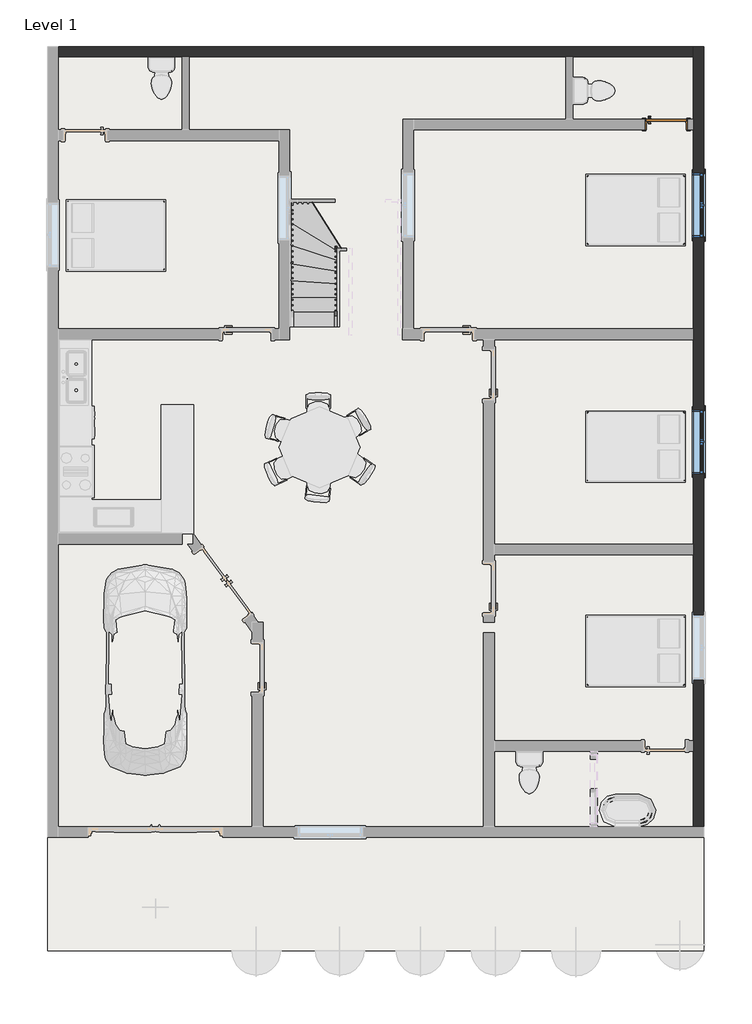
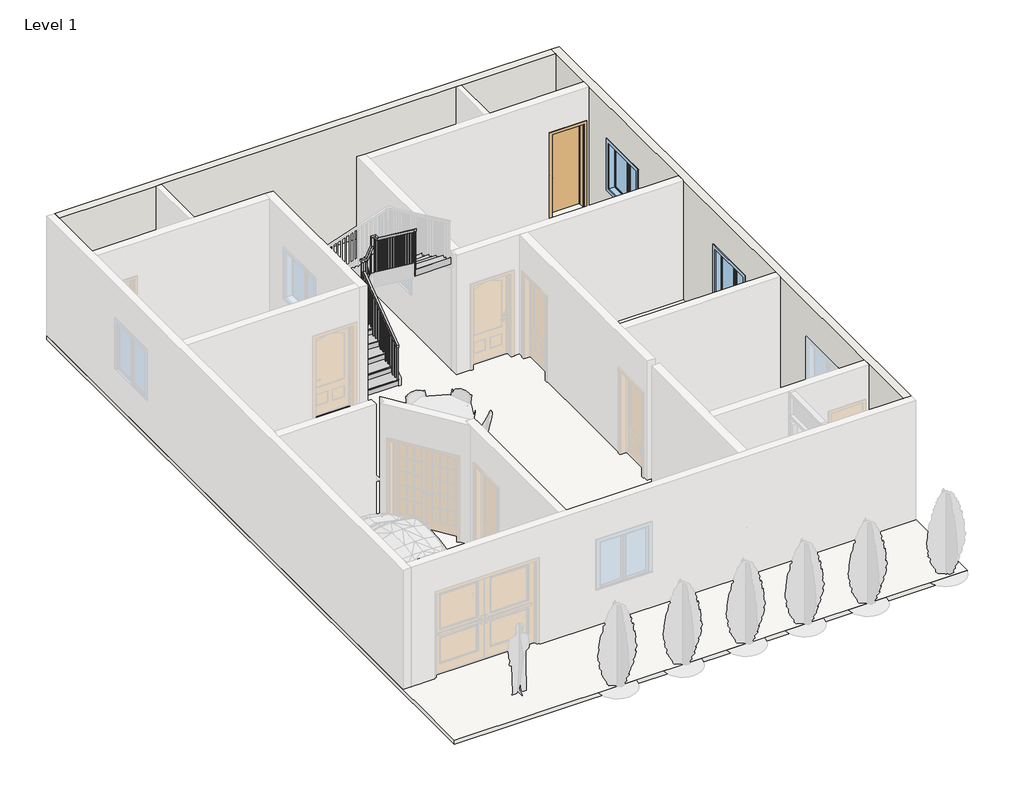
# One storey, part 2 of 3: 2 walls, 2 windows, 1 door, 1 railing, 1 slab, 1 stair flight.
"""IFC4 building model written with IfcOpenShell, lengths in millimetres."""

from ifc_helpers import new_model, si_unit, frame, origin, place, context, project, spatial, polyline, outline, extrude, faceted_brep, transform, mapped, element, save
from components import door_715cd483, stair_flight_58ce975e, window_d2c79e1c

model = new_model("IFC4")

# Units and contexts
model_context = context("Model", 3, world=origin())
ifc_project = project(units=[si_unit("LENGTHUNIT", "METRE", prefix="MILLI")], contexts=[model_context])

# Site, building, storey
site = spatial("IfcSite", under=ifc_project)
building = spatial("IfcBuilding", under=site)
storey = spatial("IfcBuildingStorey", under=building, Name="Level 1", Elevation=0.0)

# Door
placement = place(None, origin())
door_shape = door_715cd483(model_context)
element("IfcDoor", 1, ObjectType="Door-Interior-Single-Flush_Panel-Wood : 30\" x 84\"", at=placement, inside=storey, context=model_context, shape_type="MappedRepresentation", body=[
    mapped(door_shape, transform((9115.2875253, 6893.0277309, 0.0), x_axis=(1.0, 0.0, 0.0), y_axis=(0.0, 1.0, 0.0), z_axis=(0.0, 0.0, 1.0))),
])

# Railing
element("IfcRailing", 2, ObjectType="Handrail - Rectangular", at=placement, inside=storey, context=model_context, shape_type="SolidModel", body=[
    faceted_brep([(2841.0207007, 3072.6312797, 1047.851748), (2841.0207007, 3072.6312797, 984.8215118), (2891.8207007, 3072.6312797, 984.8215118), (2891.8207007, 3072.6312797, 1047.851748), (2841.0207007, 4480.7853358, 2082.1188207), (2841.0207007, 4531.5853358, 2056.4003879), (2891.8207007, 4531.5853358, 2056.4003879), (2891.8207007, 4480.7853358, 2082.1188207), (2841.0207007, 4480.7853358, 2326.0056881), (2841.0207007, 4531.5853358, 2275.2056881), (2891.8207007, 4531.5853358, 2275.2056881), (2891.8207007, 4480.7853358, 2326.0056881), (2841.0207007, 4607.7853358, 2326.0056881), (2841.0207007, 4607.7853358, 2275.2056881), (2891.8207007, 4556.9853358, 2275.2056881), (2891.8207007, 4556.9853358, 2326.0056881), (2968.0207007, 4607.7853358, 2326.0056881), (3000.34384, 4607.7853358, 2275.2056881), (3000.34384, 4556.9853358, 2275.2056881), (2968.0207007, 4556.9853358, 2326.0056881), (3095.0207007, 4607.7853358, 2597.5625884), (3145.8207007, 4607.7853358, 2586.2706121), (3145.8207007, 4556.9853358, 2586.2706121), (3095.0207007, 4556.9853358, 2597.5625884), (3095.0207007, 4607.7853358, 2827.5043941), (3145.8207007, 4607.7853358, 2776.7043941), (3145.8207007, 4556.9853358, 2776.7043941), (3095.0207007, 4556.9853358, 2827.5043941), (3222.0207007, 4607.7853358, 2827.5043941), (3222.0207007, 4607.7853358, 2776.7043941), (3171.2207007, 4556.9853358, 2776.7043941), (3171.2207007, 4556.9853358, 2827.5043941), (3222.0207007, 4480.7853358, 2827.5043941), (3222.0207007, 4463.8549082, 2776.7043941), (3171.2207007, 4463.8549082, 2776.7043941), (3171.2207007, 4480.7853358, 2827.5043941), (3222.0207007, 2913.6927876, 4002.5717223), (3171.2207007, 2913.6927876, 4002.5717223), (3171.2207007, 2913.6927876, 3939.076625), (3222.0207007, 2913.6927876, 3939.076625)], [[[0, 1, 2, 3]], [[1, 0, 4, 5]], [[2, 1, 5, 6]], [[3, 2, 6, 7]], [[0, 3, 7, 4]], [[5, 4, 8, 9]], [[6, 5, 9, 10]], [[7, 6, 10, 11]], [[4, 7, 11, 8]], [[9, 8, 12, 13]], [[10, 9, 13, 14]], [[11, 10, 14, 15]], [[8, 11, 15, 12]], [[13, 12, 16, 17]], [[14, 13, 17, 18]], [[15, 14, 18, 19]], [[12, 15, 19, 16]], [[17, 16, 20, 21]], [[18, 17, 21, 22]], [[19, 18, 22, 23]], [[16, 19, 23, 20]], [[21, 20, 24, 25]], [[22, 21, 25, 26]], [[23, 22, 26, 27]], [[20, 23, 27, 24]], [[25, 24, 28, 29]], [[26, 25, 29, 30]], [[27, 26, 30, 31]], [[24, 27, 31, 28]], [[29, 28, 32, 33]], [[30, 29, 33, 34]], [[31, 30, 34, 35]], [[28, 31, 35, 32]], [[36, 37, 38, 39]], [[33, 32, 36, 39]], [[34, 33, 39, 38]], [[35, 34, 38, 37]], [[32, 35, 37, 36]]]),
    extrude(outline(polyline([(2904.9263419, 3945.6500491), (2923.9763419, 3931.3656135), (2923.9763419, 2878.6666667), (2904.9263419, 2878.6666667), (2904.9263419, 3945.6500491)])), frame((3187.0957007, 0.0, 0.0), z_axis=(1.0, 0.0, 0.0), x_axis=(0.0, 1.0, 0.0)), (0.0, 0.0, 1.0), 19.05),
    extrude(outline(polyline([(3006.5263419, 3869.4663925), (3025.5763419, 3855.1819569), (3025.5763419, 2878.6666667), (3006.5263419, 2878.6666667), (3006.5263419, 3869.4663925)])), frame((3187.0957007, 0.0, 0.0), z_axis=(1.0, 0.0, 0.0), x_axis=(0.0, 1.0, 0.0)), (0.0, 0.0, 1.0), 19.05),
    extrude(outline(polyline([(3108.1263419, 3793.2827359), (3127.1763419, 3778.9983003), (3127.1763419, 2878.6666667), (3108.1263419, 2878.6666667), (3108.1263419, 3793.2827359)])), frame((3187.0957007, 0.0, 0.0), z_axis=(1.0, 0.0, 0.0), x_axis=(0.0, 1.0, 0.0)), (0.0, 0.0, 1.0), 19.05),
    extrude(outline(polyline([(3209.7263419, 3717.0990793), (3228.7763419, 3702.8146437), (3228.7763419, 2709.3333333), (3209.7263419, 2709.3333333), (3209.7263419, 3717.0990793)])), frame((3187.0957007, 0.0, 0.0), z_axis=(1.0, 0.0, 0.0), x_axis=(0.0, 1.0, 0.0)), (0.0, 0.0, 1.0), 19.05),
    extrude(outline(polyline([(3311.3263419, 3640.9154227), (3330.3763419, 3626.6309871), (3330.3763419, 2709.3333333), (3311.3263419, 2709.3333333), (3311.3263419, 3640.9154227)])), frame((3187.0957007, 0.0, 0.0), z_axis=(1.0, 0.0, 0.0), x_axis=(0.0, 1.0, 0.0)), (0.0, 0.0, 1.0), 19.05),
    extrude(outline(polyline([(3412.9263419, 3564.7317661), (3431.9763419, 3550.4473305), (3431.9763419, 2709.3333333), (3412.9263419, 2709.3333333), (3412.9263419, 3564.7317661)])), frame((3187.0957007, 0.0, 0.0), z_axis=(1.0, 0.0, 0.0), x_axis=(0.0, 1.0, 0.0)), (0.0, 0.0, 1.0), 19.05),
    extrude(outline(polyline([(3514.5263419, 3488.5481095), (3533.5763419, 3474.2636739), (3533.5763419, 2540.0), (3514.5263419, 2540.0), (3514.5263419, 3488.5481095)])), frame((3187.0957007, 0.0, 0.0), z_axis=(1.0, 0.0, 0.0), x_axis=(0.0, 1.0, 0.0)), (0.0, 0.0, 1.0), 19.05),
    extrude(outline(polyline([(3616.1263419, 3412.3644529), (3635.1763419, 3398.0800173), (3635.1763419, 2540.0), (3616.1263419, 2540.0), (3616.1263419, 3412.3644529)])), frame((3187.0957007, 0.0, 0.0), z_axis=(1.0, 0.0, 0.0), x_axis=(0.0, 1.0, 0.0)), (0.0, 0.0, 1.0), 19.05),
    extrude(outline(polyline([(3717.7263419, 3336.1807963), (3736.7763419, 3321.8963607), (3736.7763419, 2370.6666667), (3717.7263419, 2370.6666667), (3717.7263419, 3336.1807963)])), frame((3187.0957007, 0.0, 0.0), z_axis=(1.0, 0.0, 0.0), x_axis=(0.0, 1.0, 0.0)), (0.0, 0.0, 1.0), 19.05),
    extrude(outline(polyline([(3819.3263419, 3259.9971397), (3838.3763419, 3245.7127041), (3838.3763419, 2370.6666667), (3819.3263419, 2370.6666667), (3819.3263419, 3259.9971397)])), frame((3187.0957007, 0.0, 0.0), z_axis=(1.0, 0.0, 0.0), x_axis=(0.0, 1.0, 0.0)), (0.0, 0.0, 1.0), 19.05),
    extrude(outline(polyline([(3920.9263419, 3183.8134831), (3939.9763419, 3169.5290475), (3939.9763419, 2370.6666667), (3920.9263419, 2370.6666667), (3920.9263419, 3183.8134831)])), frame((3187.0957007, 0.0, 0.0), z_axis=(1.0, 0.0, 0.0), x_axis=(0.0, 1.0, 0.0)), (0.0, 0.0, 1.0), 19.05),
    extrude(outline(polyline([(4022.5263419, 3107.6298265), (4041.5763419, 3093.3453909), (4041.5763419, 2201.3333333), (4022.5263419, 2201.3333333), (4022.5263419, 3107.6298265)])), frame((3187.0957007, 0.0, 0.0), z_axis=(1.0, 0.0, 0.0), x_axis=(0.0, 1.0, 0.0)), (0.0, 0.0, 1.0), 19.05),
    extrude(outline(polyline([(4124.1263419, 3031.4461699), (4143.1763419, 3017.1617343), (4143.1763419, 2201.3333333), (4124.1263419, 2201.3333333), (4124.1263419, 3031.4461699)])), frame((3187.0957007, 0.0, 0.0), z_axis=(1.0, 0.0, 0.0), x_axis=(0.0, 1.0, 0.0)), (0.0, 0.0, 1.0), 19.05),
    extrude(outline(polyline([(4225.7263419, 2955.2625133), (4244.7763419, 2940.9780777), (4244.7763419, 2032.0), (4225.7263419, 2032.0), (4225.7263419, 2955.2625133)])), frame((3187.0957007, 0.0, 0.0), z_axis=(1.0, 0.0, 0.0), x_axis=(0.0, 1.0, 0.0)), (0.0, 0.0, 1.0), 19.05),
    extrude(outline(polyline([(4327.3263419, 2879.0788567), (4346.3763419, 2864.7944211), (4346.3763419, 2032.0), (4327.3263419, 2032.0), (4327.3263419, 2879.0788567)])), frame((3187.0957007, 0.0, 0.0), z_axis=(1.0, 0.0, 0.0), x_axis=(0.0, 1.0, 0.0)), (0.0, 0.0, 1.0), 19.05),
    extrude(outline(polyline([(4428.9263419, 2802.8952001), (4447.9763419, 2788.6107645), (4447.9763419, 1862.6666667), (4428.9263419, 1862.6666667), (4428.9263419, 2802.8952001)])), frame((3187.0957007, 0.0, 0.0), z_axis=(1.0, 0.0, 0.0), x_axis=(0.0, 1.0, 0.0)), (0.0, 0.0, 1.0), 19.05),
    extrude(outline(polyline([(2467.6943692, 3090.3657193), (2426.9608342, 3071.3157193), (1524.0, 3071.3157193), (1524.0, 3090.3657193), (2467.6943692, 3090.3657193)])), frame((0.0, 4572.8603358, 0.0), z_axis=(0.0, 1.0, 0.0), x_axis=(0.0, 0.0, 1.0)), (0.0, 0.0, 1.0), 19.05),
    extrude(outline(polyline([(2250.448849, 2988.7657193), (2209.7153139, 2969.7157193), (1354.6666667, 2969.7157193), (1354.6666667, 2988.7657193), (2250.448849, 2988.7657193)])), frame((0.0, 4572.8603358, 0.0), z_axis=(0.0, 1.0, 0.0), x_axis=(0.0, 0.0, 1.0)), (0.0, 0.0, 1.0), 19.05),
    extrude(outline(polyline([(4485.5062797, 2022.5560437), (4504.5562797, 2036.54797), (4504.5562797, 1016.0), (4485.5062797, 1016.0), (4485.5062797, 2022.5560437)])), frame((2856.8957007, 0.0, 0.0), z_axis=(1.0, 0.0, 0.0), x_axis=(0.0, 1.0, 0.0)), (0.0, 0.0, 1.0), 19.05),
    extrude(outline(polyline([(4383.9062797, 1947.9324369), (4402.9562797, 1961.9243632), (4402.9562797, 1016.0), (4383.9062797, 1016.0), (4383.9062797, 1947.9324369)])), frame((2856.8957007, 0.0, 0.0), z_axis=(1.0, 0.0, 0.0), x_axis=(0.0, 1.0, 0.0)), (0.0, 0.0, 1.0), 19.05),
    extrude(outline(polyline([(4282.3062797, 1873.3088301), (4301.3562797, 1887.3007564), (4301.3562797, 846.6666667), (4282.3062797, 846.6666667), (4282.3062797, 1873.3088301)])), frame((2856.8957007, 0.0, 0.0), z_axis=(1.0, 0.0, 0.0), x_axis=(0.0, 1.0, 0.0)), (0.0, 0.0, 1.0), 19.05),
    extrude(outline(polyline([(4180.7062797, 1798.6852234), (4199.7562797, 1812.6771496), (4199.7562797, 846.6666667), (4180.7062797, 846.6666667), (4180.7062797, 1798.6852234)])), frame((2856.8957007, 0.0, 0.0), z_axis=(1.0, 0.0, 0.0), x_axis=(0.0, 1.0, 0.0)), (0.0, 0.0, 1.0), 19.05),
    extrude(outline(polyline([(4079.1062797, 1724.0616166), (4098.1562797, 1738.0535428), (4098.1562797, 677.3333333), (4079.1062797, 677.3333333), (4079.1062797, 1724.0616166)])), frame((2856.8957007, 0.0, 0.0), z_axis=(1.0, 0.0, 0.0), x_axis=(0.0, 1.0, 0.0)), (0.0, 0.0, 1.0), 19.05),
    extrude(outline(polyline([(3977.5062797, 1649.4380098), (3996.5562797, 1663.429936), (3996.5562797, 677.3333333), (3977.5062797, 677.3333333), (3977.5062797, 1649.4380098)])), frame((2856.8957007, 0.0, 0.0), z_axis=(1.0, 0.0, 0.0), x_axis=(0.0, 1.0, 0.0)), (0.0, 0.0, 1.0), 19.05),
    extrude(outline(polyline([(3875.9062797, 1574.814403), (3894.9562797, 1588.8063293), (3894.9562797, 677.3333333), (3875.9062797, 677.3333333), (3875.9062797, 1574.814403)])), frame((2856.8957007, 0.0, 0.0), z_axis=(1.0, 0.0, 0.0), x_axis=(0.0, 1.0, 0.0)), (0.0, 0.0, 1.0), 19.05),
    extrude(outline(polyline([(3774.3062797, 1500.1907962), (3793.3562797, 1514.1827225), (3793.3562797, 508.0), (3774.3062797, 508.0), (3774.3062797, 1500.1907962)])), frame((2856.8957007, 0.0, 0.0), z_axis=(1.0, 0.0, 0.0), x_axis=(0.0, 1.0, 0.0)), (0.0, 0.0, 1.0), 19.05),
    extrude(outline(polyline([(3672.7062797, 1425.5671894), (3691.7562797, 1439.5591157), (3691.7562797, 508.0), (3672.7062797, 508.0), (3672.7062797, 1425.5671894)])), frame((2856.8957007, 0.0, 0.0), z_axis=(1.0, 0.0, 0.0), x_axis=(0.0, 1.0, 0.0)), (0.0, 0.0, 1.0), 19.05),
    extrude(outline(polyline([(3571.1062797, 1350.9435826), (3590.1562797, 1364.9355089), (3590.1562797, 338.6666667), (3571.1062797, 338.6666667), (3571.1062797, 1350.9435826)])), frame((2856.8957007, 0.0, 0.0), z_axis=(1.0, 0.0, 0.0), x_axis=(0.0, 1.0, 0.0)), (0.0, 0.0, 1.0), 19.05),
    extrude(outline(polyline([(3469.5062797, 1276.3199758), (3488.5562797, 1290.3119021), (3488.5562797, 338.6666667), (3469.5062797, 338.6666667), (3469.5062797, 1276.3199758)])), frame((2856.8957007, 0.0, 0.0), z_axis=(1.0, 0.0, 0.0), x_axis=(0.0, 1.0, 0.0)), (0.0, 0.0, 1.0), 19.05),
    extrude(outline(polyline([(3367.9062797, 1201.6963691), (3386.9562797, 1215.6882953), (3386.9562797, 338.6666667), (3367.9062797, 338.6666667), (3367.9062797, 1201.6963691)])), frame((2856.8957007, 0.0, 0.0), z_axis=(1.0, 0.0, 0.0), x_axis=(0.0, 1.0, 0.0)), (0.0, 0.0, 1.0), 19.05),
    extrude(outline(polyline([(3266.3062797, 1127.0727623), (3285.3562797, 1141.0646885), (3285.3562797, 169.3333333), (3266.3062797, 169.3333333), (3266.3062797, 1127.0727623)])), frame((2856.8957007, 0.0, 0.0), z_axis=(1.0, 0.0, 0.0), x_axis=(0.0, 1.0, 0.0)), (0.0, 0.0, 1.0), 19.05),
    extrude(outline(polyline([(3164.7062797, 1052.4491555), (3183.7562797, 1066.4410817), (3183.7562797, 169.3333333), (3164.7062797, 169.3333333), (3164.7062797, 1052.4491555)])), frame((2856.8957007, 0.0, 0.0), z_axis=(1.0, 0.0, 0.0), x_axis=(0.0, 1.0, 0.0)), (0.0, 0.0, 1.0), 19.05),
    extrude(outline(polyline([(3187.0957007, 4549.5763419), (3206.1457007, 4549.5763419), (3206.1457007, 4530.5263419), (3187.0957007, 4530.5263419), (3187.0957007, 4549.5763419)])), frame((0.0, 0.0, 1862.6666667), z_axis=(0.0, 0.0, 1.0), x_axis=(1.0, 0.0, 0.0)), (0.0, 0.0, 1.0), 914.0377274),
    extrude(outline(polyline([(3187.0957007, 4572.8603358), (3187.0957007, 4591.9103358), (3206.1457007, 4591.9103358), (3206.1457007, 4572.8603358), (3187.0957007, 4572.8603358)])), frame((0.0, 0.0, 1693.3333333), z_axis=(0.0, 0.0, 1.0), x_axis=(1.0, 0.0, 0.0)), (0.0, 0.0, 1.0), 1083.3710607),
    extrude(outline(polyline([(3172.2500162, 4572.8603358), (3172.2500162, 4591.9103358), (3191.3000162, 4591.9103358), (3191.3000162, 4572.8603358), (3172.2500162, 4572.8603358)])), frame((0.0, 0.0, 1693.3333333), z_axis=(0.0, 0.0, 1.0), x_axis=(1.0, 0.0, 0.0)), (0.0, 0.0, 1.0), 1083.3710607),
    extrude(outline(polyline([(2868.1157193, 4572.8603358), (2868.1157193, 4591.9103358), (2887.1657193, 4591.9103358), (2887.1657193, 4572.8603358), (2868.1157193, 4572.8603358)])), frame((0.0, 0.0, 1185.3333333), z_axis=(0.0, 0.0, 1.0), x_axis=(1.0, 0.0, 0.0)), (0.0, 0.0, 1.0), 1089.8723548),
    extrude(outline(polyline([(2875.9457007, 4572.8603358), (2856.8957007, 4572.8603358), (2856.8957007, 4591.9103358), (2875.9457007, 4591.9103358), (2875.9457007, 4572.8603358)])), frame((0.0, 0.0, 1185.3333333), z_axis=(0.0, 0.0, 1.0), x_axis=(1.0, 0.0, 0.0)), (0.0, 0.0, 1.0), 1089.8723548),
    extrude(outline(polyline([(2875.9457007, 4540.1964257), (2856.8957007, 4540.1964257), (2856.8957007, 4559.2464257), (2875.9457007, 4559.2464257), (2875.9457007, 4540.1964257)])), frame((0.0, 0.0, 1185.3333333), z_axis=(0.0, 0.0, 1.0), x_axis=(1.0, 0.0, 0.0)), (0.0, 0.0, 1.0), 1089.8723548),
    extrude(outline(polyline([(2913.6927876, 3939.076625), (2932.7427876, 3924.7921894), (2932.7427876, 2878.6666667), (2913.6927876, 2878.6666667), (2913.6927876, 3939.076625)])), frame((3187.0957007, 0.0, 0.0), z_axis=(1.0, 0.0, 0.0), x_axis=(0.0, 1.0, 0.0)), (0.0, 0.0, 1.0), 19.05),
    extrude(outline(polyline([(3072.6312797, 984.8215118), (3091.6812797, 998.8134381), (3091.6812797, 169.3333333), (3072.6312797, 169.3333333), (3072.6312797, 984.8215118)])), frame((2856.8957007, 0.0, 0.0), z_axis=(1.0, 0.0, 0.0), x_axis=(0.0, 1.0, 0.0)), (0.0, 0.0, 1.0), 19.05),
])

# Slab
element("IfcSlab", 3, ObjectType="LW Concrete on Metal Deck", at=placement, inside=storey, context=model_context, shape_type="SweptSolid", body=[
    extrude(outline(polyline([(-2573.4749747, 8363.0527309), (9821.7250253, 8363.0527309), (9821.7250253, -8713.8662612), (-2573.4749747, -8713.8662612), (-2573.4749747, 8363.0527309)])), frame((0.0, 0.0, -104.775), z_axis=(0.0, 0.0, 1.0), x_axis=(1.0, 0.0, 0.0)), (0.0, 0.0, 1.0), 104.775),
])

# Stair flight
stair_flight_shape = stair_flight_58ce975e(model_context)
element("IfcStairFlight", 4, ObjectType="2\" Tread 1\" Nosing 1/4\" Riser", at=placement, inside=storey, context=model_context, shape_type="MappedRepresentation", body=[
    mapped(stair_flight_shape, transform((0.0, 0.0, 0.0), x_axis=(1.0, 0.0, 0.0), y_axis=(0.0, 1.0, 0.0), z_axis=(0.0, 0.0, 1.0))),
])

# Walls
element("IfcWall", 5, ObjectType="Generic - 8\" Masonry", at=placement, inside=storey, context=model_context, shape_type="Brep", body=[
    faceted_brep([(-2379.7999747, 8169.3777309, 0.0), (-33.4749747, 8169.3777309, 0.0), (93.5250253, 8169.3777309, 0.0), (7218.2250253, 8169.3777309, 0.0), (7345.2250253, 8169.3777309, 0.0), (9628.0500253, 8169.3777309, 0.0), (9628.0500253, 8169.3777309, 3048.0), (7345.2250253, 8169.3777309, 3048.0), (7218.2250253, 8169.3777309, 3048.0), (93.5250253, 8169.3777309, 3048.0), (-33.4749747, 8169.3777309, 3048.0), (-2379.7999747, 8169.3777309, 3048.0), (-2379.7999747, 8363.0527309, 0.0), (-2379.7999747, 8363.0527309, 3048.0), (9628.0500253, 8363.0527309, 3048.0), (9628.0500253, 8363.0527309, 0.0)], [[[0, 1, 2, 3, 4, 5, 6, 7, 8, 9, 10, 11]], [[12, 13, 14, 15]], [[6, 5, 15, 14]], [[5, 4, 3, 2, 1, 0, 12, 15]], [[0, 11, 13, 12]], [[11, 10, 9, 8, 7, 6, 14, 13]]]),
])
element("IfcWall", 6, ObjectType="Generic - 8\" Masonry", at=placement, inside=storey, context=model_context, shape_type="Brep", body=[
    faceted_brep([(9628.0500253, 8363.0527309, 0.0), (9628.0500253, 8169.3777309, 0.0), (9628.0500253, 6991.4527309, 0.0), (9628.0500253, 6788.2527309, 0.0), (9628.0500253, 3029.0527309, 0.0), (9628.0500253, 2825.8527309, 0.0), (9628.0500253, -1034.9472691, 0.0), (9628.0500253, -1238.1472691, 0.0), (9628.0500253, -4743.3472691, 0.0), (9628.0500253, -4946.5472691, 0.0), (9628.0500253, -6368.9472691, 0.0), (9628.0500253, -6368.9472691, 3048.0), (9628.0500253, -4946.5472691, 3048.0), (9628.0500253, -4743.3472691, 3048.0), (9628.0500253, -1238.1472691, 3048.0), (9628.0500253, -1034.9472691, 3048.0), (9628.0500253, 2825.8527309, 3048.0), (9628.0500253, 3029.0527309, 3048.0), (9628.0500253, 6788.2527309, 3048.0), (9628.0500253, 6991.4527309, 3048.0), (9628.0500253, 8169.3777309, 3048.0), (9628.0500253, 8363.0527309, 3048.0), (9628.0500253, 4756.2527309, 2133.6), (9628.0500253, 4756.2527309, 914.4), (9628.0500253, 5975.4527309, 914.4), (9628.0500253, 5975.4527309, 2133.6), (9628.0500253, 285.8527309, 2133.6), (9628.0500253, 285.8527309, 914.4), (9628.0500253, 1505.0527309, 914.4), (9628.0500253, 1505.0527309, 2133.6), (9628.0500253, -3600.3472691, 2133.6), (9628.0500253, -3600.3472691, 914.4), (9628.0500253, -2381.1472691, 914.4), (9628.0500253, -2381.1472691, 2133.6), (9821.7250253, 8363.0527309, 0.0), (9821.7250253, 8363.0527309, 3048.0), (9821.7250253, -6368.9472691, 3048.0), (9821.7250253, -6368.9472691, 0.0), (9821.7250253, 4756.2527309, 2133.6), (9821.7250253, 5975.4527309, 2133.6), (9821.7250253, 5975.4527309, 914.4), (9821.7250253, 4756.2527309, 914.4), (9821.7250253, 285.8527309, 2133.6), (9821.7250253, 1505.0527309, 2133.6), (9821.7250253, 1505.0527309, 914.4), (9821.7250253, 285.8527309, 914.4), (9821.7250253, -3600.3472691, 2133.6), (9821.7250253, -2381.1472691, 2133.6), (9821.7250253, -2381.1472691, 914.4), (9821.7250253, -3600.3472691, 914.4)], [[[0, 1, 2, 3, 4, 5, 6, 7, 8, 9, 10, 11, 12, 13, 14, 15, 16, 17, 18, 19, 20, 21], [22, 23, 24, 25], [26, 27, 28, 29], [30, 31, 32, 33]], [[34, 35, 36, 37], [38, 39, 40, 41], [42, 43, 44, 45], [46, 47, 48, 49]], [[10, 9, 8, 7, 6, 5, 4, 3, 2, 1, 0, 34, 37]], [[0, 21, 35, 34]], [[11, 10, 37, 36]], [[23, 22, 38, 41]], [[24, 23, 41, 40]], [[25, 24, 40, 39]], [[22, 25, 39, 38]], [[27, 26, 42, 45]], [[28, 27, 45, 44]], [[29, 28, 44, 43]], [[26, 29, 43, 42]], [[31, 30, 46, 49]], [[32, 31, 49, 48]], [[33, 32, 48, 47]], [[30, 33, 47, 46]], [[21, 20, 19, 18, 17, 16, 15, 14, 13, 12, 11, 36, 35]]]),
])

# Windows
window_shape = window_d2c79e1c(model_context)
element("IfcWindow", 7, ObjectType="Casement Dbl with Trim : 48\" x 48\"", at=placement, inside=storey, context=model_context, shape_type="MappedRepresentation", body=[
    mapped(window_shape, transform((9705.8375253, 5365.8527309, 0.0), x_axis=(0.0, -1.0, 0.0), y_axis=(1.0, 0.0, 0.0), z_axis=(0.0, 0.0, 1.0))),
])
element("IfcWindow", 8, ObjectType="Casement Dbl with Trim : 48\" x 48\"", at=placement, inside=storey, context=model_context, shape_type="MappedRepresentation", body=[
    mapped(window_shape, transform((9705.8375253, 895.4527309, 0.0), x_axis=(0.0, -1.0, 0.0), y_axis=(1.0, 0.0, 0.0), z_axis=(0.0, 0.0, 1.0))),
])

save(model, "model.ifc")

# Revit data of these elements
# Type "Door-Interior-Single-Flush_Panel-Wood : 30\" x 84\""
#   Type Mark = "12"
#   Assembly Code = "C1020300"
#   Analytic Construction = "Wooden"
#   Thickness = 0' - 1 3/8"
#   Thermal Resistance (R) = 2.5876 (h·ft²·°F)/BTU
#   Swing Angle [instance default] = 90.00°
#   Rough Width = 2' - 8"
#   Rough Height = 7' - 1"
#   Height = 7' - 0"
#   Width = 2' - 6"
#   Heat Transfer Coefficient (U) = 0.3865 BTU/(h·ft²·°F)
#   Trim Material = Cherry
#   Panel Material = Cherry
#   Frame Material = Cherry
#   Door Handle Material = Aluminum
#   Visual Light Transmittance = 0
#   Solar Heat Gain Coefficient = 0
#   Wall Closure = (empty or 0)
#   Function = (empty or 0)
# Type "Handrail - Rectangular"
#   Assembly Code = "C2010400"
#   built-in parameter 1008612 = 0.0416667 (stored number, unit not read)
#   built-in parameter 1008611 = 0.0416667 (stored number, unit not read)
#   built-in parameter 1008609 = 0.333333 (stored number, unit not read)
#   built-in parameter 1008604 = 0.166667 (stored number, unit not read)
#   built-in parameter 1008603 = 0.166667 (stored number, unit not read)
#   Railing Height = 3' - 0"
#   built-in parameter 1008630 = 2
#   built-in parameter 1008610 = 2
#   built-in parameter 1008618 = Baluster - Square : 3/4"
# Type "LW Concrete on Metal Deck"
#   Assembly Code = "B1010"
#   Function = 0
#   Layers, outside or top first: 0' - 4" "Concrete, Lightweight" (function 1); 0' - 0 1/8" "Metal Deck" (function 1)
# Type "Generic - 8\" Masonry"
#   Assembly Code = "B2010"
#   Layers, outside or top first: 0' - 7 5/8" "Concrete Masonry Units" (function 1)
# Type "Casement Dbl with Trim : 48\" x 48\""
#   Type Mark = "10"
#   Construction Type Id = "GSP4R"
#   Assembly Code = "B2020100"
#   Analytic Construction = "1/8 in Pilkington single glazing"
#   Visual Light Transmittance = 0.9
#   Solar Heat Gain Coefficient = 0.78
#   Heat Transfer Coefficient (U) = 0.6496 BTU/(h·ft²·°F)
#   Height = 4' - 0"
#   Default Sill Height = 3' - 0"
#   Trim Projection - Ext. = 0' - 0 1/2"
#   Trim Projection - Int. = 0' - 0 3/4"
#   Trim Width - Exterior = 0' - 3 1/2"
#   Trim Width - Interior = 0' - 3 1/2"
#   Width = 4' - 0"
#   Window Inset = 0' - 0 3/4"
#   Define Thermal Properties by = 1
#   Glass Pane Material = Glass
#   Sash Material = Sash
#   Trim Exterior Material = Trim
#   Trim Interior Material = Trim
#   Wall Closure = (empty or 0)
# Element 1 (IfcDoor, "Door-Interior-Single-Flush_Panel-Wood : 30\" x 84\"")
#   Swing Angle = 90.00°
#   Phase Created = New Construction
#   Materials on its faces: "Cherry", "Aluminum"
# Element 2 (IfcRailing, "Handrail - Rectangular")
#   Phase Created = New Construction
# Element 3 (IfcSlab, "LW Concrete on Metal Deck")
#   Height Offset From Level = 0' - 0"
#   Phase Created = New Construction
#   Materials on its faces: "Metal Deck", "Concrete, Lightweight"
# Element 4 (IfcStairFlight, "2\" Tread 1\" Nosing 1/4\" Riser")
#   Phase Created = New Construction
# Elements 5, 6 (IfcWall, "Generic - 8\" Masonry")
#   Top Offset = 0' - 0"
#   Base Offset = 0' - 0"
#   Unconnected Height = 10' - 0"
#   wall height = 10' - 0"
#   Phase Created = New Construction
#   Base Constraint = Level 1
#   Materials on its faces: "Concrete Masonry Units"
# Element 7 (IfcWindow, "Casement Dbl with Trim : 48\" x 48\"")
#   Mark = "3"
#   Phase Created = New Construction
#   Materials on its faces: "Sash", "Trim", "Glass"
# Element 8 (IfcWindow, "Casement Dbl with Trim : 48\" x 48\"")
#   Mark = "4"
#   Phase Created = New Construction
#   Materials on its faces: "Sash", "Trim", "Glass"
# Materials
#   "Cherry": class "Wood", colour RGB 226 177 128, transparency 0, Description = "Prunus Serotina", Cost = 0
#   "Aluminum": class "Metal", colour RGB 247 247 247, transparency 0, Description = "Aluminum 6061", Cost = 0
#   "Concrete, Lightweight": class "Concrete", colour RGB 142 141 140, transparency 0, Description = "Lightweight concrete", Cost = 0
#   "Metal Deck": class "Metal", colour RGB 199 199 199, transparency 0, Description = "Steel, mill finish", Cost = 0
#   "Concrete Masonry Units": class "Masonry", colour RGB 227 227 227, transparency 0, Description = "Concrete masonry units", Cost = 0
#   "Glass": class "Glass", colour RGB 0 128 192, transparency 0.75, Description = "Soda Lime Glass", Cost = 0
#   "Sash": class "Wood", colour RGB 224 178 126, transparency 0
#   "Trim": class "Wood", colour RGB 224 178 126, transparency 0
